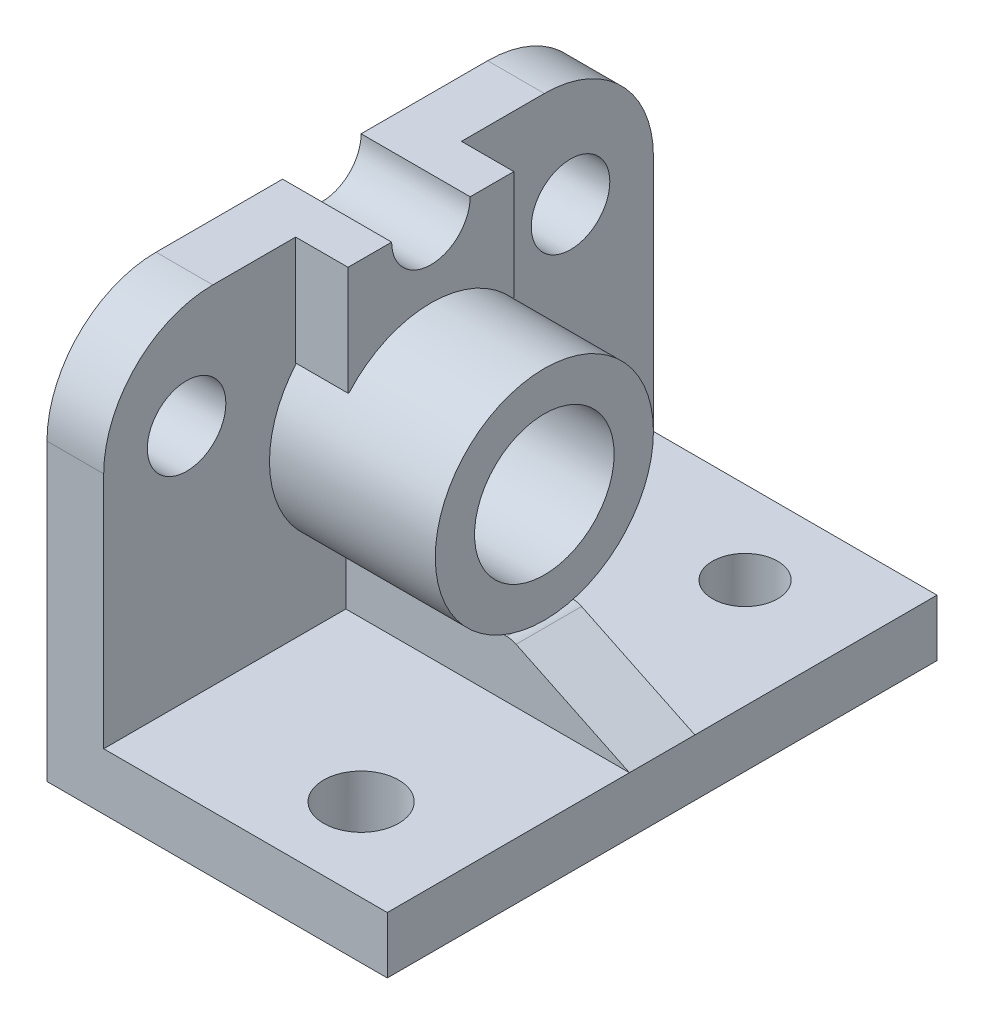
ISO-10303-21;
HEADER;
FILE_DESCRIPTION(('STEP AP214'),'2;1');
FILE_NAME('part.step','',(''),(''),'','','');
FILE_SCHEMA(('AUTOMOTIVE_DESIGN { 1 0 10303 214 1 1 1 1 }'));
ENDSEC;
DATA;
#1=APPLICATION_CONTEXT('core data for automotive mechanical design processes');
#2=APPLICATION_PROTOCOL_DEFINITION('international standard','automotive_design',2000,#1);
#3=PRODUCT_CONTEXT('',#1,'mechanical');
#4=PRODUCT('Part','Part','',(#3));
#5=PRODUCT_RELATED_PRODUCT_CATEGORY('part','',(#4));
#6=PRODUCT_DEFINITION_FORMATION('','',#4);
#7=PRODUCT_DEFINITION_CONTEXT('part definition',#1,'design');
#8=PRODUCT_DEFINITION('design','',#6,#7);
#9=PRODUCT_DEFINITION_SHAPE('','',#8);
#10=(LENGTH_UNIT() NAMED_UNIT(*) SI_UNIT(.MILLI.,.METRE.));
#11=(NAMED_UNIT(*) PLANE_ANGLE_UNIT() SI_UNIT($,.RADIAN.));
#12=(NAMED_UNIT(*) SI_UNIT($,.STERADIAN.) SOLID_ANGLE_UNIT());
#13=UNCERTAINTY_MEASURE_WITH_UNIT(LENGTH_MEASURE(1.E-05),#10,'distance_accuracy_value','');
#14=(GEOMETRIC_REPRESENTATION_CONTEXT(3) GLOBAL_UNCERTAINTY_ASSIGNED_CONTEXT((#13)) GLOBAL_UNIT_ASSIGNED_CONTEXT((#10,
#11,#12)) REPRESENTATION_CONTEXT('',''));
#15=CARTESIAN_POINT('',(0.,0.,0.));
#16=DIRECTION('',(0.,0.,1.));
#17=DIRECTION('',(1.,0.,0.));
#18=AXIS2_PLACEMENT_3D('',#15,#16,#17);
#19=CARTESIAN_POINT('',(-26.,26.,7.5));
#20=DIRECTION('',(1.,0.,0.));
#21=DIRECTION('',(0.,0.,-1.));
#22=AXIS2_PLACEMENT_3D('',#19,#20,#21);
#23=PLANE('',#22);
#24=DIRECTION('',(0.,-1.,0.));
#25=VECTOR('',#24,1.);
#26=CARTESIAN_POINT('',(-26.,26.,-7.5));
#27=LINE('',#26,#25);
#28=CARTESIAN_POINT('',(-26.,26.,-7.5));
#29=VERTEX_POINT('',#28);
#30=CARTESIAN_POINT('',(-26.,13.,-7.5));
#31=VERTEX_POINT('',#30);
#32=EDGE_CURVE('E119',#29,#31,#27,.T.);
#33=ORIENTED_EDGE('',*,*,#32,.T.);
#34=DIRECTION('',(0.,0.,-1.));
#35=VECTOR('',#34,1.);
#36=CARTESIAN_POINT('',(-26.,13.,7.5));
#37=LINE('',#36,#35);
#38=CARTESIAN_POINT('',(-26.,13.,7.5));
#39=VERTEX_POINT('',#38);
#40=EDGE_CURVE('E105',#39,#31,#37,.T.);
#41=ORIENTED_EDGE('',*,*,#40,.F.);
#42=DIRECTION('',(0.,-1.,0.));
#43=VECTOR('',#42,1.);
#44=CARTESIAN_POINT('',(-26.,26.,7.5));
#45=LINE('',#44,#43);
#46=CARTESIAN_POINT('',(-26.,26.,7.5));
#47=VERTEX_POINT('',#46);
#48=EDGE_CURVE('E108',#47,#39,#45,.T.);
#49=ORIENTED_EDGE('',*,*,#48,.F.);
#50=DIRECTION('',(0.,0.,-1.));
#51=VECTOR('',#50,1.);
#52=CARTESIAN_POINT('',(-26.,26.,7.5));
#53=LINE('',#52,#51);
#54=EDGE_CURVE('E123',#47,#29,#53,.T.);
#55=ORIENTED_EDGE('',*,*,#54,.T.);
#56=EDGE_LOOP('',(#33,#41,#49,#55));
#57=FACE_BOUND('',#56,.T.);
#58=ADVANCED_FACE('F51',(#57),#23,.F.);
#59=CARTESIAN_POINT('',(-26.,13.,7.5));
#60=DIRECTION('',(0.,1.,0.));
#61=DIRECTION('',(0.,0.,1.));
#62=AXIS2_PLACEMENT_3D('',#59,#60,#61);
#63=PLANE('',#62);
#64=DIRECTION('',(1.,0.,0.));
#65=VECTOR('',#64,1.);
#66=CARTESIAN_POINT('',(-26.,13.,-7.5));
#67=LINE('',#66,#65);
#68=CARTESIAN_POINT('',(39.,13.,-7.5));
#69=VERTEX_POINT('',#68);
#70=EDGE_CURVE('E134',#31,#69,#67,.T.);
#71=ORIENTED_EDGE('',*,*,#70,.T.);
#72=DIRECTION('',(0.,0.,-1.));
#73=VECTOR('',#72,1.);
#74=CARTESIAN_POINT('',(39.,13.,7.5));
#75=LINE('',#74,#73);
#76=CARTESIAN_POINT('',(39.,13.,7.5));
#77=VERTEX_POINT('',#76);
#78=EDGE_CURVE('E102',#77,#69,#75,.T.);
#79=ORIENTED_EDGE('',*,*,#78,.F.);
#80=DIRECTION('',(1.,0.,0.));
#81=VECTOR('',#80,1.);
#82=CARTESIAN_POINT('',(-26.,13.,7.5));
#83=LINE('',#82,#81);
#84=EDGE_CURVE('E96',#39,#77,#83,.T.);
#85=ORIENTED_EDGE('',*,*,#84,.F.);
#86=ORIENTED_EDGE('',*,*,#40,.T.);
#87=EDGE_LOOP('',(#71,#79,#85,#86));
#88=FACE_BOUND('',#87,.T.);
#89=ADVANCED_FACE('F99',(#88),#63,.F.);
#90=CARTESIAN_POINT('',(39.,13.,7.5));
#91=DIRECTION('',(-0.4338156187729,-0.9010016697591,0.));
#92=DIRECTION('',(0.9010016697591,-0.4338156187729,0.));
#93=AXIS2_PLACEMENT_3D('',#90,#91,#92);
#94=PLANE('',#93);
#95=DIRECTION('',(-0.9010016697591,0.4338156187729,0.));
#96=VECTOR('',#95,1.);
#97=CARTESIAN_POINT('',(39.,13.,-7.5));
#98=LINE('',#97,#96);
#99=CARTESIAN_POINT('',(13.0280595832709,25.5050083487955,-7.5));
#100=VERTEX_POINT('',#99);
#101=EDGE_CURVE('E131',#69,#100,#98,.T.);
#102=ORIENTED_EDGE('',*,*,#101,.T.);
#103=DIRECTION('',(0.,0.,-1.));
#104=VECTOR('',#103,1.);
#105=CARTESIAN_POINT('',(13.0280595832709,25.5050083487955,7.5));
#106=LINE('',#105,#104);
#107=CARTESIAN_POINT('',(13.0280595832709,25.5050083487955,7.5));
#108=VERTEX_POINT('',#107);
#109=EDGE_CURVE('E56',#100,#108,#106,.F.);
#110=ORIENTED_EDGE('',*,*,#109,.T.);
#111=DIRECTION('',(-0.9010016697591,0.4338156187729,0.));
#112=VECTOR('',#111,1.);
#113=CARTESIAN_POINT('',(39.,13.,7.5));
#114=LINE('',#113,#112);
#115=EDGE_CURVE('E110',#77,#108,#114,.T.);
#116=ORIENTED_EDGE('',*,*,#115,.F.);
#117=ORIENTED_EDGE('',*,*,#78,.T.);
#118=EDGE_LOOP('',(#102,#110,#116,#117));
#119=FACE_BOUND('',#118,.T.);
#120=ADVANCED_FACE('F141',(#119),#94,.F.);
#121=CARTESIAN_POINT('',(-26.,26.,7.5));
#122=DIRECTION('',(0.,-1.,0.));
#123=DIRECTION('',(0.,0.,-1.));
#124=AXIS2_PLACEMENT_3D('',#121,#122,#123);
#125=PLANE('',#124);
#126=DIRECTION('',(-1.,0.,0.));
#127=VECTOR('',#126,1.);
#128=CARTESIAN_POINT('',(-26.,26.,7.5));
#129=LINE('',#128,#127);
#130=CARTESIAN_POINT('',(10.8589814894064,26.,7.5));
#131=VERTEX_POINT('',#130);
#132=EDGE_CURVE('E113',#131,#47,#129,.T.);
#133=ORIENTED_EDGE('',*,*,#132,.F.);
#134=DIRECTION('',(0.,0.,-1.));
#135=VECTOR('',#134,1.);
#136=CARTESIAN_POINT('',(10.8589814894064,26.,7.5));
#137=LINE('',#136,#135);
#138=CARTESIAN_POINT('',(10.8589814894064,26.,-7.5));
#139=VERTEX_POINT('',#138);
#140=EDGE_CURVE('E122',#131,#139,#137,.T.);
#141=ORIENTED_EDGE('',*,*,#140,.T.);
#142=DIRECTION('',(-1.,0.,0.));
#143=VECTOR('',#142,1.);
#144=CARTESIAN_POINT('',(-26.,26.,-7.5));
#145=LINE('',#144,#143);
#146=EDGE_CURVE('E120',#139,#29,#145,.T.);
#147=ORIENTED_EDGE('',*,*,#146,.T.);
#148=ORIENTED_EDGE('',*,*,#54,.F.);
#149=EDGE_LOOP('',(#133,#141,#147,#148));
#150=FACE_BOUND('',#149,.T.);
#151=ADVANCED_FACE('F142',(#150),#125,.F.);
#152=CARTESIAN_POINT('',(0.,0.,7.5));
#153=DIRECTION('',(0.,0.,1.));
#154=DIRECTION('',(1.,0.,0.));
#155=AXIS2_PLACEMENT_3D('',#152,#153,#154);
#156=PLANE('',#155);
#157=ORIENTED_EDGE('',*,*,#115,.T.);
#158=CARTESIAN_POINT('',(10.8589814894064,21.,7.5));
#159=DIRECTION('',(0.,0.,1.));
#160=DIRECTION('',(1.,0.,0.));
#161=AXIS2_PLACEMENT_3D('',#158,#159,#160);
#162=CIRCLE('',#161,5.);
#163=EDGE_CURVE('E12',#108,#131,#162,.T.);
#164=ORIENTED_EDGE('',*,*,#163,.T.);
#165=ORIENTED_EDGE('',*,*,#132,.T.);
#166=ORIENTED_EDGE('',*,*,#48,.T.);
#167=ORIENTED_EDGE('',*,*,#84,.T.);
#168=EDGE_LOOP('',(#157,#164,#165,#166,#167));
#169=FACE_BOUND('',#168,.T.);
#170=ADVANCED_FACE('F111',(#169),#156,.T.);
#171=CARTESIAN_POINT('',(0.,0.,-7.5));
#172=DIRECTION('',(0.,0.,1.));
#173=DIRECTION('',(1.,0.,0.));
#174=AXIS2_PLACEMENT_3D('',#171,#172,#173);
#175=PLANE('',#174);
#176=ORIENTED_EDGE('',*,*,#146,.F.);
#177=CARTESIAN_POINT('',(10.8589814894064,21.,-7.5));
#178=DIRECTION('',(0.,0.,1.));
#179=DIRECTION('',(1.,0.,0.));
#180=AXIS2_PLACEMENT_3D('',#177,#178,#179);
#181=CIRCLE('',#180,5.);
#182=EDGE_CURVE('E73',#139,#100,#181,.F.);
#183=ORIENTED_EDGE('',*,*,#182,.T.);
#184=ORIENTED_EDGE('',*,*,#101,.F.);
#185=ORIENTED_EDGE('',*,*,#70,.F.);
#186=ORIENTED_EDGE('',*,*,#32,.F.);
#187=EDGE_LOOP('',(#176,#183,#184,#185,#186));
#188=FACE_BOUND('',#187,.T.);
#189=ADVANCED_FACE('F145',(#188),#175,.F.);
#190=CARTESIAN_POINT('',(10.8589814894064,21.,7.5));
#191=DIRECTION('',(0.,0.,-1.));
#192=DIRECTION('',(-1.,0.,0.));
#193=AXIS2_PLACEMENT_3D('',#190,#191,#192);
#194=CYLINDRICAL_SURFACE('',#193,5.);
#195=ORIENTED_EDGE('',*,*,#163,.F.);
#196=ORIENTED_EDGE('',*,*,#109,.F.);
#197=ORIENTED_EDGE('',*,*,#182,.F.);
#198=ORIENTED_EDGE('',*,*,#140,.F.);
#199=EDGE_LOOP('',(#195,#196,#197,#198));
#200=FACE_BOUND('',#199,.T.);
#201=ADVANCED_FACE('F52',(#200),#194,.T.);
#202=CLOSED_SHELL('',(#58,#89,#120,#151,#170,#189,#201));
#203=MANIFOLD_SOLID_BREP('B2',#202);
#204=CARTESIAN_POINT('',(-14.,67.5743346659055,0.));
#205=DIRECTION('',(0.,-1.,0.));
#206=DIRECTION('',(0.,0.,-1.));
#207=AXIS2_PLACEMENT_3D('',#204,#205,#206);
#208=PLANE('',#207);
#209=DIRECTION('',(0.,0.,1.));
#210=VECTOR('',#209,1.);
#211=CARTESIAN_POINT('',(-26.,67.5743346659055,0.));
#212=LINE('',#211,#210);
#213=CARTESIAN_POINT('',(-26.,67.5743346659055,18.7160741177888));
#214=VERTEX_POINT('',#213);
#215=CARTESIAN_POINT('',(-26.,67.5743346659055,19.));
#216=VERTEX_POINT('',#215);
#217=EDGE_CURVE('E328',#214,#216,#212,.T.);
#218=ORIENTED_EDGE('',*,*,#217,.F.);
#219=DIRECTION('',(-1.,0.,0.));
#220=VECTOR('',#219,1.);
#221=CARTESIAN_POINT('',(12.,67.5743346659055,18.7160741177888));
#222=LINE('',#221,#220);
#223=CARTESIAN_POINT('',(-14.,67.5743346659055,18.7160741177888));
#224=VERTEX_POINT('',#223);
#225=EDGE_CURVE('E329',#214,#224,#222,.F.);
#226=ORIENTED_EDGE('',*,*,#225,.T.);
#227=DIRECTION('',(0.,0.,1.));
#228=VECTOR('',#227,1.);
#229=CARTESIAN_POINT('',(-14.,67.5743346659055,0.));
#230=LINE('',#229,#228);
#231=CARTESIAN_POINT('',(-14.,67.5743346659055,19.));
#232=VERTEX_POINT('',#231);
#233=EDGE_CURVE('E313',#224,#232,#230,.T.);
#234=ORIENTED_EDGE('',*,*,#233,.T.);
#235=DIRECTION('',(-1.,0.,0.));
#236=VECTOR('',#235,1.);
#237=CARTESIAN_POINT('',(-14.,67.5743346659055,19.));
#238=LINE('',#237,#236);
#239=EDGE_CURVE('E380',#232,#216,#238,.T.);
#240=ORIENTED_EDGE('',*,*,#239,.T.);
#241=EDGE_LOOP('',(#218,#226,#234,#240));
#242=FACE_BOUND('',#241,.T.);
#243=ADVANCED_FACE('F201',(#242),#208,.T.);
#244=CARTESIAN_POINT('',(-14.,67.5743346659055,-19.));
#245=VERTEX_POINT('',#244);
#246=CARTESIAN_POINT('',(-14.,67.5743346659055,-18.7160741177888));
#247=VERTEX_POINT('',#246);
#248=EDGE_CURVE('E323',#245,#247,#230,.T.);
#249=ORIENTED_EDGE('',*,*,#248,.T.);
#250=DIRECTION('',(-1.,0.,0.));
#251=VECTOR('',#250,1.);
#252=CARTESIAN_POINT('',(12.,67.5743346659055,-18.7160741177888));
#253=LINE('',#252,#251);
#254=CARTESIAN_POINT('',(-26.,67.5743346659055,-18.7160741177888));
#255=VERTEX_POINT('',#254);
#256=EDGE_CURVE('E222',#247,#255,#253,.T.);
#257=ORIENTED_EDGE('',*,*,#256,.T.);
#258=CARTESIAN_POINT('',(-26.,67.5743346659055,-19.));
#259=VERTEX_POINT('',#258);
#260=EDGE_CURVE('E209',#259,#255,#212,.T.);
#261=ORIENTED_EDGE('',*,*,#260,.F.);
#262=DIRECTION('',(-1.,0.,0.));
#263=VECTOR('',#262,1.);
#264=CARTESIAN_POINT('',(-14.,67.5743346659055,-19.));
#265=LINE('',#264,#263);
#266=EDGE_CURVE('E378',#245,#259,#265,.T.);
#267=ORIENTED_EDGE('',*,*,#266,.F.);
#268=EDGE_LOOP('',(#249,#257,#261,#267));
#269=FACE_BOUND('',#268,.T.);
#270=ADVANCED_FACE('F525',(#269),#208,.T.);
#271=CARTESIAN_POINT('',(-26.,92.5743346659055,63.));
#272=DIRECTION('',(0.,1.,0.));
#273=DIRECTION('',(0.,0.,1.));
#274=AXIS2_PLACEMENT_3D('',#271,#272,#273);
#275=PLANE('',#274);
#276=DIRECTION('',(0.,0.,-1.));
#277=VECTOR('',#276,1.);
#278=CARTESIAN_POINT('',(-39.,92.5743346659055,63.));
#279=LINE('',#278,#277);
#280=CARTESIAN_POINT('',(-39.,92.5743346659055,-9.00000000000001));
#281=VERTEX_POINT('',#280);
#282=CARTESIAN_POINT('',(-39.,92.5743346659055,-38.));
#283=VERTEX_POINT('',#282);
#284=EDGE_CURVE('E391',#281,#283,#279,.T.);
#285=ORIENTED_EDGE('',*,*,#284,.F.);
#286=DIRECTION('',(-1.,0.,0.));
#287=VECTOR('',#286,1.);
#288=CARTESIAN_POINT('',(-14.,92.5743346659055,-9.));
#289=LINE('',#288,#287);
#290=CARTESIAN_POINT('',(-14.,92.5743346659055,-9.));
#291=VERTEX_POINT('',#290);
#292=EDGE_CURVE('E381',#291,#281,#289,.T.);
#293=ORIENTED_EDGE('',*,*,#292,.F.);
#294=DIRECTION('',(0.,0.,-1.));
#295=VECTOR('',#294,1.);
#296=CARTESIAN_POINT('',(-14.,92.5743346659055,0.));
#297=LINE('',#296,#295);
#298=CARTESIAN_POINT('',(-14.,92.5743346659055,-19.));
#299=VERTEX_POINT('',#298);
#300=EDGE_CURVE('E362',#291,#299,#297,.T.);
#301=ORIENTED_EDGE('',*,*,#300,.T.);
#302=DIRECTION('',(-1.,0.,0.));
#303=VECTOR('',#302,1.);
#304=CARTESIAN_POINT('',(-14.,92.5743346659055,-19.));
#305=LINE('',#304,#303);
#306=CARTESIAN_POINT('',(-26.,92.5743346659055,-19.));
#307=VERTEX_POINT('',#306);
#308=EDGE_CURVE('E385',#299,#307,#305,.T.);
#309=ORIENTED_EDGE('',*,*,#308,.T.);
#310=DIRECTION('',(0.,0.,-1.));
#311=VECTOR('',#310,1.);
#312=CARTESIAN_POINT('',(-26.,92.5743346659055,63.));
#313=LINE('',#312,#311);
#314=CARTESIAN_POINT('',(-26.,92.5743346659055,-38.));
#315=VERTEX_POINT('',#314);
#316=EDGE_CURVE('E395',#307,#315,#313,.T.);
#317=ORIENTED_EDGE('',*,*,#316,.T.);
#318=DIRECTION('',(-1.,0.,0.));
#319=VECTOR('',#318,1.);
#320=CARTESIAN_POINT('',(-39.,92.5743346659055,-38.));
#321=LINE('',#320,#319);
#322=EDGE_CURVE('E444',#315,#283,#321,.T.);
#323=ORIENTED_EDGE('',*,*,#322,.T.);
#324=EDGE_LOOP('',(#285,#293,#301,#309,#317,#323));
#325=FACE_BOUND('',#324,.T.);
#326=ADVANCED_FACE('F510',(#325),#275,.T.);
#327=CARTESIAN_POINT('',(0.,13.,0.));
#328=DIRECTION('',(0.,-1.,0.));
#329=DIRECTION('',(0.,0.,-1.));
#330=AXIS2_PLACEMENT_3D('',#327,#328,#329);
#331=PLANE('',#330);
#332=CARTESIAN_POINT('',(14.,13.,-44.));
#333=DIRECTION('',(0.,1.,0.));
#334=DIRECTION('',(0.,0.,1.));
#335=AXIS2_PLACEMENT_3D('',#332,#333,#334);
#336=CIRCLE('',#335,7.4725383254017);
#337=CARTESIAN_POINT('',(14.,13.,-36.5274616745983));
#338=VERTEX_POINT('',#337);
#339=EDGE_CURVE('E344',#338,#338,#336,.T.);
#340=ORIENTED_EDGE('',*,*,#339,.F.);
#341=EDGE_LOOP('',(#340));
#342=FACE_BOUND('',#341,.T.);
#343=CARTESIAN_POINT('',(14.,13.,44.));
#344=DIRECTION('',(0.,1.,0.));
#345=DIRECTION('',(0.,0.,1.));
#346=AXIS2_PLACEMENT_3D('',#343,#344,#345);
#347=CIRCLE('',#346,8.60908843550267);
#348=CARTESIAN_POINT('',(14.,13.,52.6090884355027));
#349=VERTEX_POINT('',#348);
#350=EDGE_CURVE('E331',#349,#349,#347,.T.);
#351=ORIENTED_EDGE('',*,*,#350,.F.);
#352=EDGE_LOOP('',(#351));
#353=FACE_BOUND('',#352,.T.);
#354=DIRECTION('',(0.,0.,-1.));
#355=VECTOR('',#354,1.);
#356=CARTESIAN_POINT('',(-26.,13.,0.));
#357=LINE('',#356,#355);
#358=CARTESIAN_POINT('',(-26.,13.,63.));
#359=VERTEX_POINT('',#358);
#360=CARTESIAN_POINT('',(-26.,13.,-63.));
#361=VERTEX_POINT('',#360);
#362=EDGE_CURVE('E405',#359,#361,#357,.T.);
#363=ORIENTED_EDGE('',*,*,#362,.F.);
#364=DIRECTION('',(1.,0.,0.));
#365=VECTOR('',#364,1.);
#366=CARTESIAN_POINT('',(-39.,13.,63.));
#367=LINE('',#366,#365);
#368=CARTESIAN_POINT('',(39.,13.,63.));
#369=VERTEX_POINT('',#368);
#370=EDGE_CURVE('E415',#359,#369,#367,.T.);
#371=ORIENTED_EDGE('',*,*,#370,.T.);
#372=DIRECTION('',(0.,0.,-1.));
#373=VECTOR('',#372,1.);
#374=CARTESIAN_POINT('',(39.,13.,63.));
#375=LINE('',#374,#373);
#376=CARTESIAN_POINT('',(39.,13.,-63.));
#377=VERTEX_POINT('',#376);
#378=EDGE_CURVE('E410',#369,#377,#375,.T.);
#379=ORIENTED_EDGE('',*,*,#378,.T.);
#380=DIRECTION('',(-1.,0.,0.));
#381=VECTOR('',#380,1.);
#382=CARTESIAN_POINT('',(-39.,13.,-63.));
#383=LINE('',#382,#381);
#384=EDGE_CURVE('E411',#377,#361,#383,.T.);
#385=ORIENTED_EDGE('',*,*,#384,.T.);
#386=EDGE_LOOP('',(#363,#371,#379,#385));
#387=FACE_BOUND('',#386,.T.);
#388=ADVANCED_FACE('F513',(#342,#353,#387),#331,.F.);
#389=CARTESIAN_POINT('',(39.,13.,63.));
#390=DIRECTION('',(-1.,0.,0.));
#391=DIRECTION('',(0.,0.,1.));
#392=AXIS2_PLACEMENT_3D('',#389,#390,#391);
#393=PLANE('',#392);
#394=DIRECTION('',(0.,0.,-1.));
#395=VECTOR('',#394,1.);
#396=CARTESIAN_POINT('',(39.,0.,63.));
#397=LINE('',#396,#395);
#398=CARTESIAN_POINT('',(39.,0.,63.));
#399=VERTEX_POINT('',#398);
#400=CARTESIAN_POINT('',(39.,0.,-63.));
#401=VERTEX_POINT('',#400);
#402=EDGE_CURVE('E406',#399,#401,#397,.T.);
#403=ORIENTED_EDGE('',*,*,#402,.T.);
#404=DIRECTION('',(0.,-1.,0.));
#405=VECTOR('',#404,1.);
#406=CARTESIAN_POINT('',(39.,13.,-63.));
#407=LINE('',#406,#405);
#408=EDGE_CURVE('E433',#377,#401,#407,.T.);
#409=ORIENTED_EDGE('',*,*,#408,.F.);
#410=ORIENTED_EDGE('',*,*,#378,.F.);
#411=DIRECTION('',(0.,-1.,0.));
#412=VECTOR('',#411,1.);
#413=CARTESIAN_POINT('',(39.,13.,63.));
#414=LINE('',#413,#412);
#415=EDGE_CURVE('E420',#369,#399,#414,.T.);
#416=ORIENTED_EDGE('',*,*,#415,.T.);
#417=EDGE_LOOP('',(#403,#409,#410,#416));
#418=FACE_BOUND('',#417,.T.);
#419=ADVANCED_FACE('F484',(#418),#393,.F.);
#420=CARTESIAN_POINT('',(-39.,13.,-63.));
#421=DIRECTION('',(0.,0.,1.));
#422=DIRECTION('',(1.,0.,0.));
#423=AXIS2_PLACEMENT_3D('',#420,#421,#422);
#424=PLANE('',#423);
#425=DIRECTION('',(0.,-1.,0.));
#426=VECTOR('',#425,1.);
#427=CARTESIAN_POINT('',(-39.,13.,-63.));
#428=LINE('',#427,#426);
#429=CARTESIAN_POINT('',(-39.,67.5743346659055,-63.));
#430=VERTEX_POINT('',#429);
#431=CARTESIAN_POINT('',(-39.,0.,-63.));
#432=VERTEX_POINT('',#431);
#433=EDGE_CURVE('E431',#430,#432,#428,.T.);
#434=ORIENTED_EDGE('',*,*,#433,.F.);
#435=DIRECTION('',(-1.,0.,0.));
#436=VECTOR('',#435,1.);
#437=CARTESIAN_POINT('',(-26.,67.5743346659055,-63.));
#438=LINE('',#437,#436);
#439=CARTESIAN_POINT('',(-26.,67.5743346659055,-63.));
#440=VERTEX_POINT('',#439);
#441=EDGE_CURVE('E448',#430,#440,#438,.F.);
#442=ORIENTED_EDGE('',*,*,#441,.T.);
#443=DIRECTION('',(0.,-1.,0.));
#444=VECTOR('',#443,1.);
#445=CARTESIAN_POINT('',(-26.,92.5743346659055,-63.));
#446=LINE('',#445,#444);
#447=EDGE_CURVE('E399',#440,#361,#446,.T.);
#448=ORIENTED_EDGE('',*,*,#447,.T.);
#449=ORIENTED_EDGE('',*,*,#384,.F.);
#450=ORIENTED_EDGE('',*,*,#408,.T.);
#451=DIRECTION('',(-1.,0.,0.));
#452=VECTOR('',#451,1.);
#453=CARTESIAN_POINT('',(-39.,0.,-63.));
#454=LINE('',#453,#452);
#455=EDGE_CURVE('E419',#401,#432,#454,.T.);
#456=ORIENTED_EDGE('',*,*,#455,.T.);
#457=EDGE_LOOP('',(#434,#442,#448,#449,#450,#456));
#458=FACE_BOUND('',#457,.T.);
#459=ADVANCED_FACE('F481',(#458),#424,.F.);
#460=CARTESIAN_POINT('',(-39.,13.,63.));
#461=DIRECTION('',(1.,0.,0.));
#462=DIRECTION('',(0.,0.,-1.));
#463=AXIS2_PLACEMENT_3D('',#460,#461,#462);
#464=PLANE('',#463);
#465=CARTESIAN_POINT('',(-39.,67.5743346659055,44.));
#466=DIRECTION('',(1.,0.,0.));
#467=DIRECTION('',(0.,0.,-1.));
#468=AXIS2_PLACEMENT_3D('',#465,#466,#467);
#469=CIRCLE('',#468,9.00000000000001);
#470=CARTESIAN_POINT('',(-39.,67.5743346659055,35.));
#471=VERTEX_POINT('',#470);
#472=EDGE_CURVE('E357',#471,#471,#469,.T.);
#473=ORIENTED_EDGE('',*,*,#472,.T.);
#474=EDGE_LOOP('',(#473));
#475=FACE_BOUND('',#474,.T.);
#476=CARTESIAN_POINT('',(-39.,67.5743346659055,-44.));
#477=DIRECTION('',(1.,0.,0.));
#478=DIRECTION('',(0.,0.,-1.));
#479=AXIS2_PLACEMENT_3D('',#476,#477,#478);
#480=CIRCLE('',#479,9.00000000000001);
#481=CARTESIAN_POINT('',(-39.,67.5743346659055,-53.));
#482=VERTEX_POINT('',#481);
#483=EDGE_CURVE('E350',#482,#482,#480,.T.);
#484=ORIENTED_EDGE('',*,*,#483,.T.);
#485=EDGE_LOOP('',(#484));
#486=FACE_BOUND('',#485,.T.);
#487=CARTESIAN_POINT('',(-39.,92.5743346659055,38.));
#488=VERTEX_POINT('',#487);
#489=CARTESIAN_POINT('',(-39.,92.5743346659055,8.99999999999999));
#490=VERTEX_POINT('',#489);
#491=EDGE_CURVE('E396',#488,#490,#279,.T.);
#492=ORIENTED_EDGE('',*,*,#491,.T.);
#493=CARTESIAN_POINT('',(-39.,92.5743346659055,0.));
#494=DIRECTION('',(-1.,0.,0.));
#495=DIRECTION('',(0.,0.,1.));
#496=AXIS2_PLACEMENT_3D('',#493,#494,#495);
#497=CIRCLE('',#496,9.);
#498=EDGE_CURVE('E359',#281,#490,#497,.T.);
#499=ORIENTED_EDGE('',*,*,#498,.F.);
#500=ORIENTED_EDGE('',*,*,#284,.T.);
#501=CARTESIAN_POINT('',(-39.,67.5743346659055,-38.));
#502=DIRECTION('',(1.,0.,0.));
#503=DIRECTION('',(0.,0.,-1.));
#504=AXIS2_PLACEMENT_3D('',#501,#502,#503);
#505=CIRCLE('',#504,25.);
#506=EDGE_CURVE('E449',#283,#430,#505,.F.);
#507=ORIENTED_EDGE('',*,*,#506,.T.);
#508=ORIENTED_EDGE('',*,*,#433,.T.);
#509=DIRECTION('',(0.,0.,1.));
#510=VECTOR('',#509,1.);
#511=CARTESIAN_POINT('',(-39.,0.,63.));
#512=LINE('',#511,#510);
#513=CARTESIAN_POINT('',(-39.,0.,63.));
#514=VERTEX_POINT('',#513);
#515=EDGE_CURVE('E421',#432,#514,#512,.T.);
#516=ORIENTED_EDGE('',*,*,#515,.T.);
#517=DIRECTION('',(0.,-1.,0.));
#518=VECTOR('',#517,1.);
#519=CARTESIAN_POINT('',(-39.,13.,63.));
#520=LINE('',#519,#518);
#521=CARTESIAN_POINT('',(-39.,67.5743346659055,63.));
#522=VERTEX_POINT('',#521);
#523=EDGE_CURVE('E429',#522,#514,#520,.T.);
#524=ORIENTED_EDGE('',*,*,#523,.F.);
#525=CARTESIAN_POINT('',(-39.,67.5743346659055,38.));
#526=DIRECTION('',(1.,0.,0.));
#527=DIRECTION('',(0.,0.,-1.));
#528=AXIS2_PLACEMENT_3D('',#525,#526,#527);
#529=CIRCLE('',#528,25.);
#530=EDGE_CURVE('E437',#522,#488,#529,.F.);
#531=ORIENTED_EDGE('',*,*,#530,.T.);
#532=EDGE_LOOP('',(#492,#499,#500,#507,#508,#516,#524,#531));
#533=FACE_BOUND('',#532,.T.);
#534=ADVANCED_FACE('F476',(#475,#486,#533),#464,.F.);
#535=CARTESIAN_POINT('',(-39.,13.,63.));
#536=DIRECTION('',(0.,0.,-1.));
#537=DIRECTION('',(-1.,0.,0.));
#538=AXIS2_PLACEMENT_3D('',#535,#536,#537);
#539=PLANE('',#538);
#540=DIRECTION('',(0.,1.,0.));
#541=VECTOR('',#540,1.);
#542=CARTESIAN_POINT('',(-26.,0.,63.));
#543=LINE('',#542,#541);
#544=CARTESIAN_POINT('',(-26.,67.5743346659055,63.));
#545=VERTEX_POINT('',#544);
#546=EDGE_CURVE('E392',#359,#545,#543,.T.);
#547=ORIENTED_EDGE('',*,*,#546,.T.);
#548=DIRECTION('',(-1.,0.,0.));
#549=VECTOR('',#548,1.);
#550=CARTESIAN_POINT('',(-39.,67.5743346659055,63.));
#551=LINE('',#550,#549);
#552=EDGE_CURVE('E436',#545,#522,#551,.T.);
#553=ORIENTED_EDGE('',*,*,#552,.T.);
#554=ORIENTED_EDGE('',*,*,#523,.T.);
#555=DIRECTION('',(1.,0.,0.));
#556=VECTOR('',#555,1.);
#557=CARTESIAN_POINT('',(-39.,0.,63.));
#558=LINE('',#557,#556);
#559=EDGE_CURVE('E412',#514,#399,#558,.T.);
#560=ORIENTED_EDGE('',*,*,#559,.T.);
#561=ORIENTED_EDGE('',*,*,#415,.F.);
#562=ORIENTED_EDGE('',*,*,#370,.F.);
#563=EDGE_LOOP('',(#547,#553,#554,#560,#561,#562));
#564=FACE_BOUND('',#563,.T.);
#565=ADVANCED_FACE('F470',(#564),#539,.F.);
#566=CARTESIAN_POINT('',(0.,0.,0.));
#567=DIRECTION('',(0.,-1.,0.));
#568=DIRECTION('',(0.,0.,-1.));
#569=AXIS2_PLACEMENT_3D('',#566,#567,#568);
#570=PLANE('',#569);
#571=CARTESIAN_POINT('',(14.,0.,-44.));
#572=DIRECTION('',(0.,-1.,0.));
#573=DIRECTION('',(0.,0.,-1.));
#574=AXIS2_PLACEMENT_3D('',#571,#572,#573);
#575=CIRCLE('',#574,7.4725383254017);
#576=CARTESIAN_POINT('',(14.,0.,-51.4725383254017));
#577=VERTEX_POINT('',#576);
#578=EDGE_CURVE('E352',#577,#577,#575,.T.);
#579=ORIENTED_EDGE('',*,*,#578,.F.);
#580=EDGE_LOOP('',(#579));
#581=FACE_BOUND('',#580,.T.);
#582=CARTESIAN_POINT('',(14.,0.,44.));
#583=DIRECTION('',(0.,-1.,0.));
#584=DIRECTION('',(0.,0.,-1.));
#585=AXIS2_PLACEMENT_3D('',#582,#583,#584);
#586=CIRCLE('',#585,8.60908843550267);
#587=CARTESIAN_POINT('',(14.,0.,35.3909115644973));
#588=VERTEX_POINT('',#587);
#589=EDGE_CURVE('E343',#588,#588,#586,.T.);
#590=ORIENTED_EDGE('',*,*,#589,.F.);
#591=EDGE_LOOP('',(#590));
#592=FACE_BOUND('',#591,.T.);
#593=ORIENTED_EDGE('',*,*,#515,.F.);
#594=ORIENTED_EDGE('',*,*,#455,.F.);
#595=ORIENTED_EDGE('',*,*,#402,.F.);
#596=ORIENTED_EDGE('',*,*,#559,.F.);
#597=EDGE_LOOP('',(#593,#594,#595,#596));
#598=FACE_BOUND('',#597,.T.);
#599=ADVANCED_FACE('F463',(#581,#592,#598),#570,.T.);
#600=CARTESIAN_POINT('',(-26.,0.,0.));
#601=DIRECTION('',(-1.,0.,0.));
#602=DIRECTION('',(0.,0.,1.));
#603=AXIS2_PLACEMENT_3D('',#600,#601,#602);
#604=PLANE('',#603);
#605=CARTESIAN_POINT('',(-26.,51.,0.));
#606=DIRECTION('',(1.,0.,0.));
#607=DIRECTION('',(0.,0.,-1.));
#608=AXIS2_PLACEMENT_3D('',#605,#606,#607);
#609=CIRCLE('',#608,25.);
#610=EDGE_CURVE('E216',#214,#255,#609,.T.);
#611=ORIENTED_EDGE('',*,*,#610,.F.);
#612=ORIENTED_EDGE('',*,*,#217,.T.);
#613=DIRECTION('',(0.,1.,0.));
#614=VECTOR('',#613,1.);
#615=CARTESIAN_POINT('',(-26.,0.,19.));
#616=LINE('',#615,#614);
#617=CARTESIAN_POINT('',(-26.,92.5743346659055,19.));
#618=VERTEX_POINT('',#617);
#619=EDGE_CURVE('E390',#216,#618,#616,.T.);
#620=ORIENTED_EDGE('',*,*,#619,.T.);
#621=CARTESIAN_POINT('',(-26.,92.5743346659055,38.));
#622=VERTEX_POINT('',#621);
#623=EDGE_CURVE('E400',#622,#618,#313,.T.);
#624=ORIENTED_EDGE('',*,*,#623,.F.);
#625=CARTESIAN_POINT('',(-26.,67.5743346659055,38.));
#626=DIRECTION('',(-1.,0.,0.));
#627=DIRECTION('',(0.,0.,1.));
#628=AXIS2_PLACEMENT_3D('',#625,#626,#627);
#629=CIRCLE('',#628,25.);
#630=EDGE_CURVE('E442',#622,#545,#629,.F.);
#631=ORIENTED_EDGE('',*,*,#630,.T.);
#632=ORIENTED_EDGE('',*,*,#546,.F.);
#633=ORIENTED_EDGE('',*,*,#362,.T.);
#634=ORIENTED_EDGE('',*,*,#447,.F.);
#635=CARTESIAN_POINT('',(-26.,67.5743346659055,-38.));
#636=DIRECTION('',(-1.,0.,0.));
#637=DIRECTION('',(0.,0.,1.));
#638=AXIS2_PLACEMENT_3D('',#635,#636,#637);
#639=CIRCLE('',#638,25.);
#640=EDGE_CURVE('E451',#440,#315,#639,.F.);
#641=ORIENTED_EDGE('',*,*,#640,.T.);
#642=ORIENTED_EDGE('',*,*,#316,.F.);
#643=DIRECTION('',(0.,-1.,0.));
#644=VECTOR('',#643,1.);
#645=CARTESIAN_POINT('',(-26.,0.,-19.));
#646=LINE('',#645,#644);
#647=EDGE_CURVE('E372',#307,#259,#646,.T.);
#648=ORIENTED_EDGE('',*,*,#647,.T.);
#649=ORIENTED_EDGE('',*,*,#260,.T.);
#650=EDGE_LOOP('',(#611,#612,#620,#624,#631,#632,#633,#634,#641,#642,#648,#649));
#651=FACE_BOUND('',#650,.T.);
#652=CARTESIAN_POINT('',(-26.,67.5743346659055,44.));
#653=DIRECTION('',(1.,0.,0.));
#654=DIRECTION('',(0.,0.,-1.));
#655=AXIS2_PLACEMENT_3D('',#652,#653,#654);
#656=CIRCLE('',#655,9.00000000000001);
#657=CARTESIAN_POINT('',(-26.,67.5743346659055,35.));
#658=VERTEX_POINT('',#657);
#659=EDGE_CURVE('E347',#658,#658,#656,.T.);
#660=ORIENTED_EDGE('',*,*,#659,.F.);
#661=EDGE_LOOP('',(#660));
#662=FACE_BOUND('',#661,.T.);
#663=CARTESIAN_POINT('',(-26.,67.5743346659055,-44.));
#664=DIRECTION('',(1.,0.,0.));
#665=DIRECTION('',(0.,0.,-1.));
#666=AXIS2_PLACEMENT_3D('',#663,#664,#665);
#667=CIRCLE('',#666,9.00000000000001);
#668=CARTESIAN_POINT('',(-26.,67.5743346659055,-53.));
#669=VERTEX_POINT('',#668);
#670=EDGE_CURVE('E351',#669,#669,#667,.T.);
#671=ORIENTED_EDGE('',*,*,#670,.F.);
#672=EDGE_LOOP('',(#671));
#673=FACE_BOUND('',#672,.T.);
#674=ADVANCED_FACE('F467',(#651,#662,#673),#604,.F.);
#675=DIRECTION('',(-1.,0.,0.));
#676=VECTOR('',#675,1.);
#677=CARTESIAN_POINT('',(-14.,92.5743346659055,9.));
#678=LINE('',#677,#676);
#679=CARTESIAN_POINT('',(-14.,92.5743346659055,9.));
#680=VERTEX_POINT('',#679);
#681=EDGE_CURVE('E375',#680,#490,#678,.T.);
#682=ORIENTED_EDGE('',*,*,#681,.T.);
#683=ORIENTED_EDGE('',*,*,#491,.F.);
#684=DIRECTION('',(-1.,0.,0.));
#685=VECTOR('',#684,1.);
#686=CARTESIAN_POINT('',(-26.,92.5743346659055,38.));
#687=LINE('',#686,#685);
#688=EDGE_CURVE('E441',#488,#622,#687,.F.);
#689=ORIENTED_EDGE('',*,*,#688,.T.);
#690=ORIENTED_EDGE('',*,*,#623,.T.);
#691=DIRECTION('',(-1.,0.,0.));
#692=VECTOR('',#691,1.);
#693=CARTESIAN_POINT('',(-14.,92.5743346659055,19.));
#694=LINE('',#693,#692);
#695=CARTESIAN_POINT('',(-14.,92.5743346659055,19.));
#696=VERTEX_POINT('',#695);
#697=EDGE_CURVE('E374',#696,#618,#694,.T.);
#698=ORIENTED_EDGE('',*,*,#697,.F.);
#699=EDGE_CURVE('E368',#696,#680,#297,.T.);
#700=ORIENTED_EDGE('',*,*,#699,.T.);
#701=EDGE_LOOP('',(#682,#683,#689,#690,#698,#700));
#702=FACE_BOUND('',#701,.T.);
#703=ADVANCED_FACE('F498',(#702),#275,.T.);
#704=CARTESIAN_POINT('',(-39.,67.5743346659055,38.));
#705=DIRECTION('',(1.,0.,0.));
#706=DIRECTION('',(0.,0.,-1.));
#707=AXIS2_PLACEMENT_3D('',#704,#705,#706);
#708=CYLINDRICAL_SURFACE('',#707,25.);
#709=ORIENTED_EDGE('',*,*,#630,.F.);
#710=ORIENTED_EDGE('',*,*,#688,.F.);
#711=ORIENTED_EDGE('',*,*,#530,.F.);
#712=ORIENTED_EDGE('',*,*,#552,.F.);
#713=EDGE_LOOP('',(#709,#710,#711,#712));
#714=FACE_BOUND('',#713,.T.);
#715=ADVANCED_FACE('F491',(#714),#708,.T.);
#716=CARTESIAN_POINT('',(-26.,67.5743346659055,-38.));
#717=DIRECTION('',(1.,0.,0.));
#718=DIRECTION('',(0.,0.,-1.));
#719=AXIS2_PLACEMENT_3D('',#716,#717,#718);
#720=CYLINDRICAL_SURFACE('',#719,25.);
#721=ORIENTED_EDGE('',*,*,#640,.F.);
#722=ORIENTED_EDGE('',*,*,#441,.F.);
#723=ORIENTED_EDGE('',*,*,#506,.F.);
#724=ORIENTED_EDGE('',*,*,#322,.F.);
#725=EDGE_LOOP('',(#721,#722,#723,#724));
#726=FACE_BOUND('',#725,.T.);
#727=ADVANCED_FACE('F203',(#726),#720,.T.);
#728=CARTESIAN_POINT('',(-14.,92.5743346659055,0.));
#729=DIRECTION('',(-1.,0.,0.));
#730=DIRECTION('',(0.,0.,1.));
#731=AXIS2_PLACEMENT_3D('',#728,#729,#730);
#732=CYLINDRICAL_SURFACE('',#731,9.);
#733=ORIENTED_EDGE('',*,*,#292,.T.);
#734=ORIENTED_EDGE('',*,*,#498,.T.);
#735=ORIENTED_EDGE('',*,*,#681,.F.);
#736=CARTESIAN_POINT('',(-14.,92.5743346659055,0.));
#737=DIRECTION('',(-1.,0.,0.));
#738=DIRECTION('',(0.,0.,1.));
#739=AXIS2_PLACEMENT_3D('',#736,#737,#738);
#740=CIRCLE('',#739,9.);
#741=EDGE_CURVE('E361',#291,#680,#740,.T.);
#742=ORIENTED_EDGE('',*,*,#741,.F.);
#743=EDGE_LOOP('',(#733,#734,#735,#742));
#744=FACE_BOUND('',#743,.T.);
#745=ADVANCED_FACE('F502',(#744),#732,.F.);
#746=CARTESIAN_POINT('',(-14.,0.,19.));
#747=DIRECTION('',(0.,0.,1.));
#748=DIRECTION('',(0.,-1.,0.));
#749=AXIS2_PLACEMENT_3D('',#746,#747,#748);
#750=PLANE('',#749);
#751=ORIENTED_EDGE('',*,*,#619,.F.);
#752=ORIENTED_EDGE('',*,*,#239,.F.);
#753=DIRECTION('',(0.,1.,0.));
#754=VECTOR('',#753,1.);
#755=CARTESIAN_POINT('',(-14.,0.,19.));
#756=LINE('',#755,#754);
#757=EDGE_CURVE('E318',#232,#696,#756,.T.);
#758=ORIENTED_EDGE('',*,*,#757,.T.);
#759=ORIENTED_EDGE('',*,*,#697,.T.);
#760=EDGE_LOOP('',(#751,#752,#758,#759));
#761=FACE_BOUND('',#760,.T.);
#762=ADVANCED_FACE('F536',(#761),#750,.T.);
#763=CARTESIAN_POINT('',(-14.,0.,-19.));
#764=DIRECTION('',(0.,0.,-1.));
#765=DIRECTION('',(-1.,0.,0.));
#766=AXIS2_PLACEMENT_3D('',#763,#764,#765);
#767=PLANE('',#766);
#768=ORIENTED_EDGE('',*,*,#647,.F.);
#769=ORIENTED_EDGE('',*,*,#308,.F.);
#770=DIRECTION('',(0.,-1.,0.));
#771=VECTOR('',#770,1.);
#772=CARTESIAN_POINT('',(-14.,0.,-19.));
#773=LINE('',#772,#771);
#774=EDGE_CURVE('E322',#299,#245,#773,.T.);
#775=ORIENTED_EDGE('',*,*,#774,.T.);
#776=ORIENTED_EDGE('',*,*,#266,.T.);
#777=EDGE_LOOP('',(#768,#769,#775,#776));
#778=FACE_BOUND('',#777,.T.);
#779=ADVANCED_FACE('F538',(#778),#767,.T.);
#780=CARTESIAN_POINT('',(-14.,0.,0.));
#781=DIRECTION('',(-1.,0.,0.));
#782=DIRECTION('',(0.,0.,1.));
#783=AXIS2_PLACEMENT_3D('',#780,#781,#782);
#784=PLANE('',#783);
#785=CARTESIAN_POINT('',(-14.,51.,0.));
#786=DIRECTION('',(-1.,0.,0.));
#787=DIRECTION('',(0.,0.,1.));
#788=AXIS2_PLACEMENT_3D('',#785,#786,#787);
#789=CIRCLE('',#788,25.);
#790=EDGE_CURVE('E47',#247,#224,#789,.F.);
#791=ORIENTED_EDGE('',*,*,#790,.F.);
#792=ORIENTED_EDGE('',*,*,#248,.F.);
#793=ORIENTED_EDGE('',*,*,#774,.F.);
#794=ORIENTED_EDGE('',*,*,#300,.F.);
#795=ORIENTED_EDGE('',*,*,#741,.T.);
#796=ORIENTED_EDGE('',*,*,#699,.F.);
#797=ORIENTED_EDGE('',*,*,#757,.F.);
#798=ORIENTED_EDGE('',*,*,#233,.F.);
#799=EDGE_LOOP('',(#791,#792,#793,#794,#795,#796,#797,#798));
#800=FACE_BOUND('',#799,.T.);
#801=ADVANCED_FACE('F317',(#800),#784,.F.);
#802=CARTESIAN_POINT('',(-51.,67.5743346659055,-44.));
#803=DIRECTION('',(1.,0.,0.));
#804=DIRECTION('',(0.,0.,-1.));
#805=AXIS2_PLACEMENT_3D('',#802,#803,#804);
#806=CYLINDRICAL_SURFACE('',#805,9.00000000000001);
#807=ORIENTED_EDGE('',*,*,#670,.T.);
#808=EDGE_LOOP('',(#807));
#809=FACE_BOUND('',#808,.T.);
#810=ORIENTED_EDGE('',*,*,#483,.F.);
#811=EDGE_LOOP('',(#810));
#812=FACE_BOUND('',#811,.T.);
#813=ADVANCED_FACE('F643',(#809,#812),#806,.F.);
#814=CARTESIAN_POINT('',(-51.,67.5743346659055,44.));
#815=DIRECTION('',(1.,0.,0.));
#816=DIRECTION('',(0.,0.,-1.));
#817=AXIS2_PLACEMENT_3D('',#814,#815,#816);
#818=CYLINDRICAL_SURFACE('',#817,9.00000000000001);
#819=ORIENTED_EDGE('',*,*,#659,.T.);
#820=EDGE_LOOP('',(#819));
#821=FACE_BOUND('',#820,.T.);
#822=ORIENTED_EDGE('',*,*,#472,.F.);
#823=EDGE_LOOP('',(#822));
#824=FACE_BOUND('',#823,.T.);
#825=ADVANCED_FACE('F659',(#821,#824),#818,.F.);
#826=CARTESIAN_POINT('',(14.,-12.,44.));
#827=DIRECTION('',(0.,1.,0.));
#828=DIRECTION('',(0.,0.,1.));
#829=AXIS2_PLACEMENT_3D('',#826,#827,#828);
#830=CYLINDRICAL_SURFACE('',#829,8.60908843550267);
#831=ORIENTED_EDGE('',*,*,#589,.T.);
#832=EDGE_LOOP('',(#831));
#833=FACE_BOUND('',#832,.T.);
#834=ORIENTED_EDGE('',*,*,#350,.T.);
#835=EDGE_LOOP('',(#834));
#836=FACE_BOUND('',#835,.T.);
#837=ADVANCED_FACE('F670',(#833,#836),#830,.F.);
#838=CARTESIAN_POINT('',(14.,-12.,-44.));
#839=DIRECTION('',(0.,1.,0.));
#840=DIRECTION('',(0.,0.,1.));
#841=AXIS2_PLACEMENT_3D('',#838,#839,#840);
#842=CYLINDRICAL_SURFACE('',#841,7.4725383254017);
#843=ORIENTED_EDGE('',*,*,#578,.T.);
#844=EDGE_LOOP('',(#843));
#845=FACE_BOUND('',#844,.T.);
#846=ORIENTED_EDGE('',*,*,#339,.T.);
#847=EDGE_LOOP('',(#846));
#848=FACE_BOUND('',#847,.T.);
#849=ADVANCED_FACE('F460',(#845,#848),#842,.F.);
#850=CARTESIAN_POINT('',(12.,51.,0.));
#851=DIRECTION('',(-1.,0.,0.));
#852=DIRECTION('',(0.,0.,1.));
#853=AXIS2_PLACEMENT_3D('',#850,#851,#852);
#854=CYLINDRICAL_SURFACE('',#853,25.);
#855=ORIENTED_EDGE('',*,*,#225,.F.);
#856=ORIENTED_EDGE('',*,*,#610,.T.);
#857=ORIENTED_EDGE('',*,*,#256,.F.);
#858=ORIENTED_EDGE('',*,*,#790,.T.);
#859=EDGE_LOOP('',(#855,#856,#857,#858));
#860=FACE_BOUND('',#859,.T.);
#861=CARTESIAN_POINT('',(12.,51.,0.));
#862=DIRECTION('',(1.,0.,0.));
#863=DIRECTION('',(0.,0.,-1.));
#864=AXIS2_PLACEMENT_3D('',#861,#862,#863);
#865=CIRCLE('',#864,25.);
#866=CARTESIAN_POINT('',(12.,51.,-25.));
#867=VERTEX_POINT('',#866);
#868=EDGE_CURVE('E334',#867,#867,#865,.T.);
#869=ORIENTED_EDGE('',*,*,#868,.F.);
#870=EDGE_LOOP('',(#869));
#871=FACE_BOUND('',#870,.T.);
#872=ADVANCED_FACE('F333',(#860,#871),#854,.T.);
#873=CARTESIAN_POINT('',(12.,51.,0.));
#874=DIRECTION('',(1.,0.,0.));
#875=DIRECTION('',(0.,0.,-1.));
#876=AXIS2_PLACEMENT_3D('',#873,#874,#875);
#877=PLANE('',#876);
#878=CARTESIAN_POINT('',(12.,51.,0.));
#879=DIRECTION('',(1.,0.,0.));
#880=DIRECTION('',(0.,0.,-1.));
#881=AXIS2_PLACEMENT_3D('',#878,#879,#880);
#882=CIRCLE('',#881,16.);
#883=CARTESIAN_POINT('',(12.,51.,-16.));
#884=VERTEX_POINT('',#883);
#885=EDGE_CURVE('E739',#884,#884,#882,.T.);
#886=ORIENTED_EDGE('',*,*,#885,.F.);
#887=EDGE_LOOP('',(#886));
#888=FACE_BOUND('',#887,.T.);
#889=ORIENTED_EDGE('',*,*,#868,.T.);
#890=EDGE_LOOP('',(#889));
#891=FACE_BOUND('',#890,.T.);
#892=ADVANCED_FACE('F699',(#888,#891),#877,.T.);
#893=CARTESIAN_POINT('',(-26.,51.,0.));
#894=DIRECTION('',(1.,0.,0.));
#895=DIRECTION('',(0.,0.,-1.));
#896=AXIS2_PLACEMENT_3D('',#893,#894,#895);
#897=CYLINDRICAL_SURFACE('',#896,16.);
#898=CARTESIAN_POINT('',(-26.,51.,0.));
#899=DIRECTION('',(1.,0.,0.));
#900=DIRECTION('',(0.,0.,-1.));
#901=AXIS2_PLACEMENT_3D('',#898,#899,#900);
#902=CIRCLE('',#901,16.);
#903=CARTESIAN_POINT('',(-26.,51.,-16.));
#904=VERTEX_POINT('',#903);
#905=EDGE_CURVE('E737',#904,#904,#902,.T.);
#906=ORIENTED_EDGE('',*,*,#905,.F.);
#907=EDGE_LOOP('',(#906));
#908=FACE_BOUND('',#907,.T.);
#909=ORIENTED_EDGE('',*,*,#885,.T.);
#910=EDGE_LOOP('',(#909));
#911=FACE_BOUND('',#910,.T.);
#912=ADVANCED_FACE('F709',(#908,#911),#897,.F.);
#913=CARTESIAN_POINT('',(-26.,51.,0.));
#914=DIRECTION('',(1.,0.,0.));
#915=DIRECTION('',(0.,0.,-1.));
#916=AXIS2_PLACEMENT_3D('',#913,#914,#915);
#917=PLANE('',#916);
#918=ORIENTED_EDGE('',*,*,#905,.T.);
#919=EDGE_LOOP('',(#918));
#920=FACE_BOUND('',#919,.T.);
#921=ADVANCED_FACE('F717',(#920),#917,.T.);
#922=CLOSED_SHELL('',(#243,#270,#326,#388,#419,#459,#534,#565,#599,#674,#703,#715,#727,#745,
#762,#779,#801,#813,#825,#837,#849,#872,#892,#912,#921));
#923=MANIFOLD_SOLID_BREP('B6',#922);
#924=ADVANCED_BREP_SHAPE_REPRESENTATION('',(#18,#203,#923),#14);
#925=SHAPE_DEFINITION_REPRESENTATION(#9,#924);
ENDSEC;
END-ISO-10303-21;
